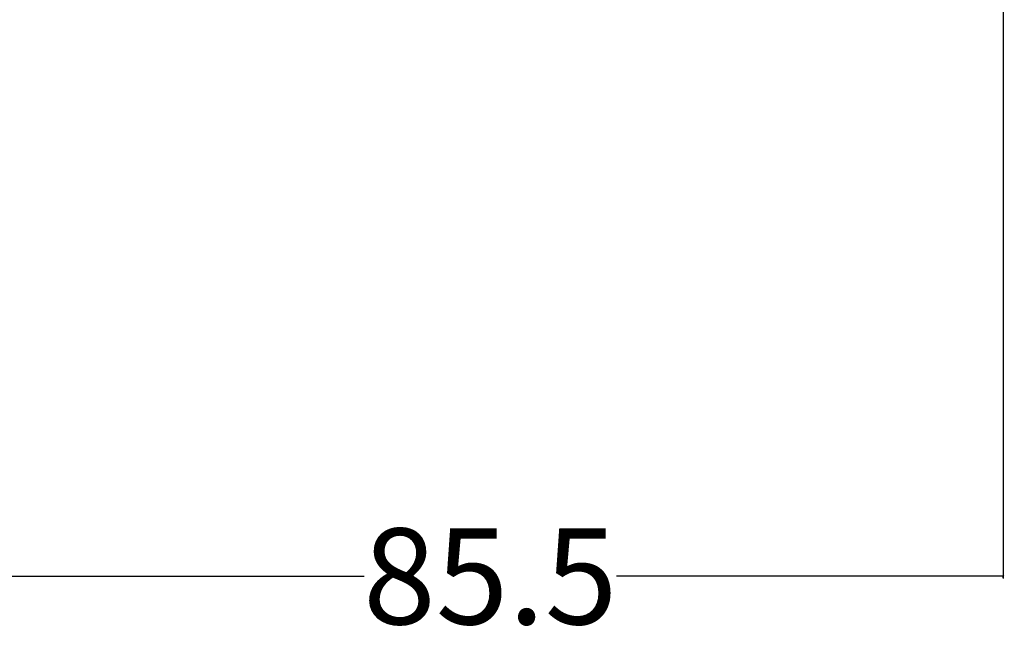
# Model space of a CAD drawing. Units: inches. Extents: x -48 to 50072, y 0 to 21068.
# Tile 32 of 75: x 467 to 549, y 161 to 213. Entities that reach past the tile are written whole.
import ezdxf

# ---------------------------------------------------------------- set-up
doc = ezdxf.new("R2010")
doc.units = ezdxf.units.IN
doc.header["$MEASUREMENT"] = 0
doc.layers.add('A-ANNO-DIMS', color=2, linetype='Continuous', lineweight=18)
doc.styles.get("Standard").update_dxf_attribs({"font": 'arial.ttf'})
doc.dimstyles.get("Standard").update_dxf_attribs({"dimtxt": 8, "dimasz": 0.18, "dimexe": 0.18, "dimexo": 0.0625, "dimgap": 0.09, "dimtad": 0, "dimtih": 1, "dimtoh": 1, "dimdec": 1, "dimzin": 0, "dimdsep": 46, "dimlunit": 4, "dimtxsty": 'Standard', "dimblk": 'ARCHTICK', "dimcen": 0.09, "dimadec": 0, "dimazin": 0, "dimtfac": 1, "dimtdec": 1, "dimtofl": 0, "dimtmove": 0, "dimatfit": 3, "dimldrblk": 'ARCHTICK', "dimfxl": 1, "dimtolj": 1, "dimtzin": 0, "dimarcsym": 0})

# ---------------------------------------------------------------- blocks, each defined once
blk = doc.blocks.new('_ArchTick')
at = {"color": 0, "linetype": 'ByBlock', "const_width": 0.15}
blk.add_lwpolyline([(-0.5, -0.5), (0.5, 0.5)], dxfattribs=at)
blk = doc.blocks.new('*D119')
at = {"layer": 'A-ANNO-DIMS', "color": 0, "lineweight": -2, "transparency": 16777216}
for p, q in [((463.517, 451.012), (463.517, 165.945)), ((549.017, 451.012), (549.017, 165.945)), ((463.517, 166.125), (495.752, 166.125)), ((549.017, 166.125), (516.783, 166.125))]:
    blk.add_line(p, q, dxfattribs=at)
at = {"layer": 'Defpoints', "color": 0, "transparency": 16777216}
for p in [(463.517, 451.075), (549.017, 451.075), (549.017, 166.125)]:
    blk.add_point(p, dxfattribs=at)
at = {"layer": 'A-ANNO-DIMS', "color": 0, "lineweight": -2, "transparency": 16777216, "xscale": 0.18, "yscale": 0.18, "zscale": 0.18, "rotation": 180}
blk.add_blockref('_ArchTick', (463.517, 166.125), dxfattribs=at)
at = {"layer": 'A-ANNO-DIMS', "color": 0, "lineweight": -2, "transparency": 16777216, "xscale": 0.18, "yscale": 0.18, "zscale": 0.18}
blk.add_blockref('_ArchTick', (549.017, 166.125), dxfattribs=at)
at = {"layer": 'A-ANNO-DIMS', "color": 0, "transparency": 16777216, "insert": (506.267, 166.125), "char_height": 8, "attachment_point": 5}
blk.add_mtext('\\A1;85.5', dxfattribs=at)

msp = doc.modelspace()

# ---------------------------------------------------------------- dimensions: what is measured, and where the dimension line sits
at = {"layer": 'A-ANNO-DIMS'}
dim = msp.add_linear_dim(base=(549.017, 166.125), p1=(463.517, 451.075), p2=(549.017, 451.075), dimstyle='Standard', override={"dimdec": 1, "dimlfac": 1, "dimrnd": 0, "dimzin": 0, "dimdsep": 46, "dimlunit": 2}, dxfattribs=at)
dim.commit()
dim.dimension.update_dxf_attribs({"geometry": '*D119', "text_midpoint": (506.267, 166.125)})

doc.saveas('drawing.dxf')
